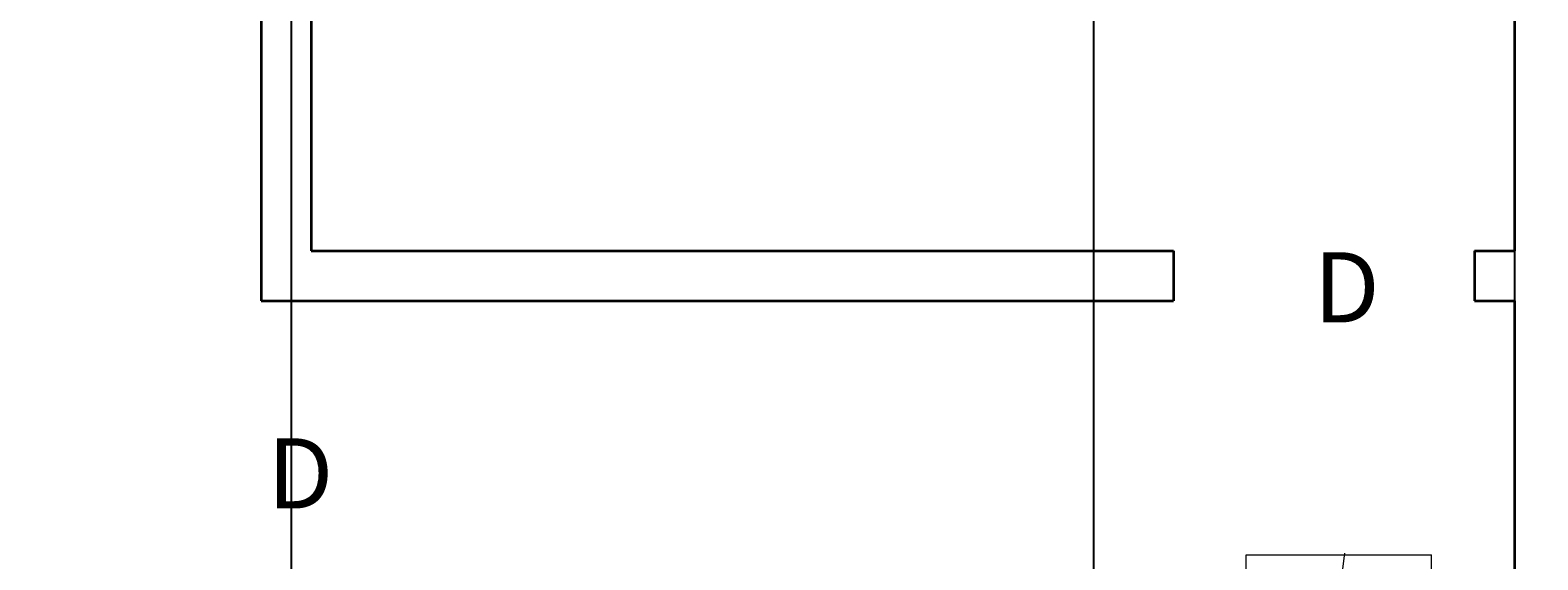
# Model space of a CAD drawing. Units: inches. Extents: x 3731 to 4318, y 1310 to 2388.
# Tile 21 of 57: x 4086 to 4237, y 1502 to 1554. Entities that reach past the tile are written whole.
import ezdxf

# ---------------------------------------------------------------- set-up
doc = ezdxf.new("R2010")
doc.units = ezdxf.units.IN
for name, color, linetype, lineweight in [('A-ANNO-DIMS', 2, 'Continuous', 18), ('A-ANNO-TEXT', 7, 'Continuous', 18), ('A-FURN', 8, 'Continuous', 13), ('A-WALL', 7, 'Continuous', 35)]:
    doc.layers.add(name, color=color, linetype=linetype, lineweight=lineweight)
doc.styles.get("Standard").update_dxf_attribs({"font": 'arial.ttf'})
doc.dimstyles.get("Standard").update_dxf_attribs({"dimtxt": 0.18, "dimasz": 0.18, "dimexe": 0.18, "dimexo": 0.0625, "dimgap": 0.09, "dimtad": 0, "dimtih": 1, "dimtoh": 1, "dimdec": 4, "dimzin": 0, "dimdsep": 46, "dimtxsty": 'Standard', "dimcen": 0.09, "dimadec": 0, "dimazin": 0, "dimtfac": 1, "dimtdec": 4, "dimtofl": 0, "dimtmove": 0, "dimatfit": 3, "dimfxl": 1, "dimtolj": 1, "dimtzin": 0, "dimarcsym": 0})

# ---------------------------------------------------------------- blocks, each defined once
blk = doc.blocks.new('A$C200C7901')
for p, q in [((2, 2.3334), (2.5, 2.3334)), ((2.5, 1.8834), (2.5, 2.3334)), ((2, 1.8834), (2.5, 1.8834))]:
    blk.add_line(p, q)
at = {"linetype": 'ByBlock'}
blk.add_line((2.2464, 2.0911), (2.5044, 2.1228), dxfattribs=at)
blk = doc.blocks.new('*D32')
at = {"layer": 'A-ANNO-DIMS', "color": 0, "lineweight": -2, "transparency": 16777216}
for p, q in [((4269.21, 1592.32), (4269.21, 1310.25)), ((3835.21, 1359.32), (3835.21, 1310.25)), ((3835.39, 1310.43), (4051.92, 1310.43)), ((4269.03, 1310.43), (4052.5, 1310.43))]:
    blk.add_line(p, q, dxfattribs=at)
at = {"layer": 'A-ANNO-DIMS', "color": 0, "transparency": 16777216}
for points in [[(3835.39, 1310.46), (3835.39, 1310.4), (3835.21, 1310.43)], [(4269.03, 1310.46), (4269.03, 1310.4), (4269.21, 1310.43)]]:
    blk.add_solid(points, dxfattribs=at)
at = {"layer": 'Defpoints', "color": 0, "transparency": 16777216}
for p in [(4269.21, 1592.38), (3835.21, 1359.38), (4269.21, 1310.43)]:
    blk.add_point(p, dxfattribs=at)
at = {"layer": 'A-ANNO-DIMS', "color": 0, "transparency": 16777216, "insert": (4052.21, 1310.43), "char_height": 0.18, "attachment_point": 5}
blk.add_mtext('\\A1;434', dxfattribs=at)
blk = doc.blocks.new('*D46')
at = {"layer": 'A-ANNO-DIMS', "color": 0, "lineweight": -2, "transparency": 16777216}
for p, q in [((4112.21, 1854.32), (4112.21, 1310.25)), ((4192.21, 1854.32), (4192.21, 1310.25)), ((4112.39, 1310.43), (4151.99, 1310.43)), ((4192.03, 1310.43), (4152.43, 1310.43))]:
    blk.add_line(p, q, dxfattribs=at)
at = {"layer": 'A-ANNO-DIMS', "color": 0, "transparency": 16777216}
for points in [[(4112.39, 1310.46), (4112.39, 1310.4), (4112.21, 1310.43)], [(4192.03, 1310.46), (4192.03, 1310.4), (4192.21, 1310.43)]]:
    blk.add_solid(points, dxfattribs=at)
at = {"layer": 'Defpoints', "color": 0, "transparency": 16777216}
for p in [(4112.21, 1854.38), (4192.21, 1854.38), (4192.21, 1310.43)]:
    blk.add_point(p, dxfattribs=at)
at = {"layer": 'A-ANNO-DIMS', "color": 0, "transparency": 16777216, "insert": (4152.21, 1310.43), "char_height": 0.18, "attachment_point": 5}
blk.add_mtext('\\A1;80', dxfattribs=at)
blk = doc.blocks.new('*D47')
at = {"layer": 'A-ANNO-DIMS', "color": 0, "lineweight": -2, "transparency": 16777216}
for p, q in [((4192.21, 1854.32), (4192.21, 1310.25)), ((4234.21, 1854.32), (4234.21, 1310.25)), ((4192.39, 1310.43), (4212.99, 1310.43)), ((4234.03, 1310.43), (4213.43, 1310.43))]:
    blk.add_line(p, q, dxfattribs=at)
at = {"layer": 'A-ANNO-DIMS', "color": 0, "transparency": 16777216}
for points in [[(4192.39, 1310.46), (4192.39, 1310.4), (4192.21, 1310.43)], [(4234.03, 1310.46), (4234.03, 1310.4), (4234.21, 1310.43)]]:
    blk.add_solid(points, dxfattribs=at)
at = {"layer": 'Defpoints', "color": 0, "transparency": 16777216}
for p in [(4192.21, 1854.38), (4234.21, 1854.38), (4234.21, 1310.43)]:
    blk.add_point(p, dxfattribs=at)
at = {"layer": 'A-ANNO-DIMS', "color": 0, "transparency": 16777216, "insert": (4213.21, 1310.43), "char_height": 0.18, "attachment_point": 5}
blk.add_mtext('\\A1;42', dxfattribs=at)

msp = doc.modelspace()

# ---------------------------------------------------------------- linework, layer by layer
at = {"layer": 'A-WALL'}
for p, q in [((4109.21, 1597.38), (4109.21, 1532.38)), ((4114.21, 1592.38), (4114.21, 1532.38)), ((4234.21, 1592.38), (4234.21, 1532.38)), ((4109.21, 1532.38), (4109.21, 1527.38)), ((4114.21, 1532.38), (4200.21, 1532.38)), ((4200.21, 1532.38), (4200.21, 1527.38)), ((4230.21, 1532.38), (4230.21, 1527.38)), ((4230.21, 1532.38), (4234.21, 1532.38)), ((4109.21, 1527.38), (4200.21, 1527.38)), ((4230.21, 1527.38), (4234.21, 1527.38)), ((4234.21, 1527.38), (4234.21, 1364.38))]:
    msp.add_line(p, q, dxfattribs=at)

# ---------------------------------------------------------------- block references
at = {"layer": 'A-FURN', "xscale": -41.1071563136412, "yscale": 41.1071563136412, "zscale": 41.1071563136412, "rotation": 270}
msp.add_blockref('A$C200C7901', (4130.02, 1399.26), dxfattribs=at)

# ---------------------------------------------------------------- texts
at = {"layer": 'A-ANNO-TEXT', "char_height": 7, "attachment_point": 1}
for insert in [(4214.19, 1532.22), (4109.84, 1513.66)]:
    msp.add_mtext_dynamic_manual_height_columns('D', width=10.4564, gutter_width=12.5, heights=[0], dxfattribs=dict(at, insert=insert))

# ---------------------------------------------------------------- dimensions: what is measured, and where the dimension line sits
at = {"layer": 'A-ANNO-DIMS'}
for base, p1, p2, picture, middle in [((4192.21, 1310.43), (4112.21, 1854.38), (4192.21, 1854.38), '*D46', (4152.21, 1310.43)), ((4234.21, 1310.43), (4192.21, 1854.38), (4234.21, 1854.38), '*D47', (4213.21, 1310.43)), ((4269.21, 1310.43), (3835.21, 1359.38), (4269.21, 1592.38), '*D32', (4052.21, 1310.43))]:
    dim = msp.add_linear_dim(base=base, p1=p1, p2=p2, dimstyle='Standard', override={"dimdec": 0, "dimlfac": 1, "dimrnd": 0, "dimzin": 0, "dimdsep": 46, "dimlunit": 2}, dxfattribs=at)
    dim.commit()
    dim.dimension.update_dxf_attribs({"geometry": picture, "text_midpoint": middle})

doc.saveas('drawing.dxf')
